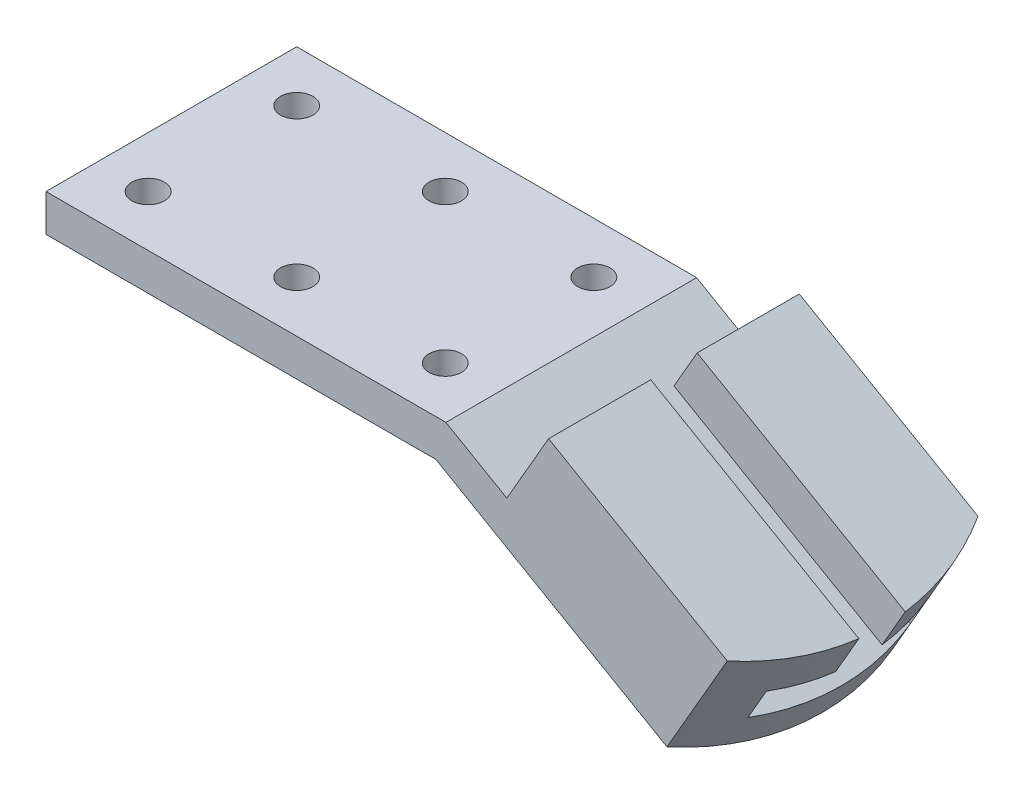
ISO-10303-21;
HEADER;
FILE_DESCRIPTION(('STEP AP214'),'2;1');
FILE_NAME('part.step','',(''),(''),'','','');
FILE_SCHEMA(('AUTOMOTIVE_DESIGN { 1 0 10303 214 1 1 1 1 }'));
ENDSEC;
DATA;
#1=APPLICATION_CONTEXT('core data for automotive mechanical design processes');
#2=APPLICATION_PROTOCOL_DEFINITION('international standard','automotive_design',2000,#1);
#3=PRODUCT_CONTEXT('',#1,'mechanical');
#4=PRODUCT('Part','Part','',(#3));
#5=PRODUCT_RELATED_PRODUCT_CATEGORY('part','',(#4));
#6=PRODUCT_DEFINITION_FORMATION('','',#4);
#7=PRODUCT_DEFINITION_CONTEXT('part definition',#1,'design');
#8=PRODUCT_DEFINITION('design','',#6,#7);
#9=PRODUCT_DEFINITION_SHAPE('','',#8);
#10=(LENGTH_UNIT() NAMED_UNIT(*) SI_UNIT(.MILLI.,.METRE.));
#11=(NAMED_UNIT(*) PLANE_ANGLE_UNIT() SI_UNIT($,.RADIAN.));
#12=(NAMED_UNIT(*) SI_UNIT($,.STERADIAN.) SOLID_ANGLE_UNIT());
#13=UNCERTAINTY_MEASURE_WITH_UNIT(LENGTH_MEASURE(1.E-05),#10,'distance_accuracy_value','');
#14=(GEOMETRIC_REPRESENTATION_CONTEXT(3) GLOBAL_UNCERTAINTY_ASSIGNED_CONTEXT((#13)) GLOBAL_UNIT_ASSIGNED_CONTEXT((#10,
#11,#12)) REPRESENTATION_CONTEXT('',''));
#15=CARTESIAN_POINT('',(0.,0.,0.));
#16=DIRECTION('',(0.,0.,1.));
#17=DIRECTION('',(1.,0.,0.));
#18=AXIS2_PLACEMENT_3D('',#15,#16,#17);
#19=CARTESIAN_POINT('',(25.0000000000001,43.301270189222,27.));
#20=DIRECTION('',(-0.500000000000001,-0.866025403784438,0.));
#21=DIRECTION('',(0.866025403784438,-0.500000000000001,0.));
#22=AXIS2_PLACEMENT_3D('',#19,#20,#21);
#23=PLANE('',#22);
#24=DIRECTION('',(0.866025403784439,-0.5,0.));
#25=VECTOR('',#24,1.);
#26=CARTESIAN_POINT('',(97.5262794416288,1.4282032302755,17.5));
#27=LINE('',#26,#25);
#28=CARTESIAN_POINT('',(99.2583302491977,0.428203230275488,17.5));
#29=VERTEX_POINT('',#28);
#30=CARTESIAN_POINT('',(141.664845078879,-24.055209522035,17.5));
#31=VERTEX_POINT('',#30);
#32=EDGE_CURVE('E246',#29,#31,#27,.T.);
#33=ORIENTED_EDGE('',*,*,#32,.T.);
#34=CARTESIAN_POINT('',(99.2583302491977,0.428203230275488,0.));
#35=DIRECTION('',(-0.500000000000001,-0.866025403784438,0.));
#36=DIRECTION('',(0.866025403784438,-0.500000000000001,0.));
#37=AXIS2_PLACEMENT_3D('',#34,#35,#36);
#38=CIRCLE('',#37,52.);
#39=CARTESIAN_POINT('',(141.664845078879,-24.055209522035,-17.5));
#40=VERTEX_POINT('',#39);
#41=EDGE_CURVE('E220',#31,#40,#38,.F.);
#42=ORIENTED_EDGE('',*,*,#41,.T.);
#43=DIRECTION('',(0.866025403784439,-0.5,0.));
#44=VECTOR('',#43,1.);
#45=CARTESIAN_POINT('',(97.5262794416288,1.4282032302755,-17.5));
#46=LINE('',#45,#44);
#47=CARTESIAN_POINT('',(99.2583302491977,0.428203230275488,-17.5));
#48=VERTEX_POINT('',#47);
#49=EDGE_CURVE('E245',#48,#40,#46,.T.);
#50=ORIENTED_EDGE('',*,*,#49,.F.);
#51=DIRECTION('',(0.,0.,-1.));
#52=VECTOR('',#51,1.);
#53=CARTESIAN_POINT('',(99.2583302491977,0.428203230275481,27.));
#54=LINE('',#53,#52);
#55=CARTESIAN_POINT('',(99.2583302491977,0.428203230275481,-27.));
#56=VERTEX_POINT('',#55);
#57=EDGE_CURVE('E168',#48,#56,#54,.T.);
#58=ORIENTED_EDGE('',*,*,#57,.T.);
#59=DIRECTION('',(-0.866025403784438,0.500000000000001,0.));
#60=VECTOR('',#59,1.);
#61=CARTESIAN_POINT('',(25.0000000000001,43.301270189222,-27.));
#62=LINE('',#61,#60);
#63=CARTESIAN_POINT('',(86.143593539449,8.,-27.));
#64=VERTEX_POINT('',#63);
#65=EDGE_CURVE('E146',#56,#64,#62,.T.);
#66=ORIENTED_EDGE('',*,*,#65,.T.);
#67=DIRECTION('',(0.,0.,-1.));
#68=VECTOR('',#67,1.);
#69=CARTESIAN_POINT('',(86.143593539449,8.,27.));
#70=LINE('',#69,#68);
#71=CARTESIAN_POINT('',(86.143593539449,8.,27.));
#72=VERTEX_POINT('',#71);
#73=EDGE_CURVE('E169',#72,#64,#70,.T.);
#74=ORIENTED_EDGE('',*,*,#73,.F.);
#75=DIRECTION('',(-0.866025403784438,0.500000000000001,0.));
#76=VECTOR('',#75,1.);
#77=CARTESIAN_POINT('',(25.0000000000001,43.301270189222,27.));
#78=LINE('',#77,#76);
#79=CARTESIAN_POINT('',(99.2583302491977,0.428203230275481,27.));
#80=VERTEX_POINT('',#79);
#81=EDGE_CURVE('E103',#80,#72,#78,.T.);
#82=ORIENTED_EDGE('',*,*,#81,.F.);
#83=EDGE_CURVE('E172',#80,#29,#54,.T.);
#84=ORIENTED_EDGE('',*,*,#83,.T.);
#85=EDGE_LOOP('',(#33,#42,#50,#58,#66,#74,#82,#84));
#86=FACE_BOUND('',#85,.T.);
#87=ADVANCED_FACE('F41',(#86),#23,.F.);
#88=CARTESIAN_POINT('',(101.526279441629,8.35640646055095,17.5));
#89=DIRECTION('',(0.5,0.866025403784439,0.));
#90=DIRECTION('',(-0.866025403784439,0.5,0.));
#91=AXIS2_PLACEMENT_3D('',#88,#89,#90);
#92=PLANE('',#91);
#93=DIRECTION('',(0.866025403784439,-0.5,0.));
#94=VECTOR('',#93,1.);
#95=CARTESIAN_POINT('',(101.526279441629,8.35640646055095,5.));
#96=LINE('',#95,#94);
#97=CARTESIAN_POINT('',(103.258330249198,7.35640646055095,5.));
#98=VERTEX_POINT('',#97);
#99=CARTESIAN_POINT('',(148.082988641649,-18.5231221286641,5.));
#100=VERTEX_POINT('',#99);
#101=EDGE_CURVE('E232',#98,#100,#96,.T.);
#102=ORIENTED_EDGE('',*,*,#101,.T.);
#103=CARTESIAN_POINT('',(103.258330249198,7.35640646055096,0.));
#104=DIRECTION('',(0.5,0.866025403784439,0.));
#105=DIRECTION('',(-0.866025403784439,0.5,0.));
#106=AXIS2_PLACEMENT_3D('',#103,#104,#105);
#107=CIRCLE('',#106,52.);
#108=CARTESIAN_POINT('',(145.664845078879,-17.1270062917595,17.5));
#109=VERTEX_POINT('',#108);
#110=EDGE_CURVE('E230',#100,#109,#107,.F.);
#111=ORIENTED_EDGE('',*,*,#110,.T.);
#112=DIRECTION('',(0.866025403784439,-0.5,0.));
#113=VECTOR('',#112,1.);
#114=CARTESIAN_POINT('',(101.526279441629,8.35640646055095,17.5));
#115=LINE('',#114,#113);
#116=CARTESIAN_POINT('',(103.258330249198,7.35640646055095,17.5));
#117=VERTEX_POINT('',#116);
#118=EDGE_CURVE('E221',#117,#109,#115,.T.);
#119=ORIENTED_EDGE('',*,*,#118,.F.);
#120=DIRECTION('',(0.,0.,1.));
#121=VECTOR('',#120,1.);
#122=CARTESIAN_POINT('',(103.258330249198,7.35640646055095,27.));
#123=LINE('',#122,#121);
#124=EDGE_CURVE('E149',#98,#117,#123,.T.);
#125=ORIENTED_EDGE('',*,*,#124,.F.);
#126=EDGE_LOOP('',(#102,#111,#119,#125));
#127=FACE_BOUND('',#126,.T.);
#128=ADVANCED_FACE('F348',(#127),#92,.F.);
#129=CARTESIAN_POINT('',(101.526279441629,8.35640646055095,-17.5));
#130=DIRECTION('',(0.5,0.866025403784439,0.));
#131=DIRECTION('',(-0.866025403784439,0.5,0.));
#132=AXIS2_PLACEMENT_3D('',#129,#130,#131);
#133=PLANE('',#132);
#134=DIRECTION('',(0.866025403784439,-0.5,0.));
#135=VECTOR('',#134,1.);
#136=CARTESIAN_POINT('',(101.526279441629,8.35640646055095,-17.5));
#137=LINE('',#136,#135);
#138=CARTESIAN_POINT('',(103.258330249198,7.35640646055095,-17.5));
#139=VERTEX_POINT('',#138);
#140=CARTESIAN_POINT('',(145.664845078879,-17.1270062917595,-17.5));
#141=VERTEX_POINT('',#140);
#142=EDGE_CURVE('E238',#139,#141,#137,.T.);
#143=ORIENTED_EDGE('',*,*,#142,.T.);
#144=CARTESIAN_POINT('',(103.258330249198,7.35640646055096,0.));
#145=DIRECTION('',(0.5,0.866025403784439,0.));
#146=DIRECTION('',(-0.866025403784439,0.5,0.));
#147=AXIS2_PLACEMENT_3D('',#144,#145,#146);
#148=CIRCLE('',#147,52.);
#149=CARTESIAN_POINT('',(148.082988641649,-18.5231221286641,-5.));
#150=VERTEX_POINT('',#149);
#151=EDGE_CURVE('E209',#141,#150,#148,.F.);
#152=ORIENTED_EDGE('',*,*,#151,.T.);
#153=DIRECTION('',(0.866025403784439,-0.5,0.));
#154=VECTOR('',#153,1.);
#155=CARTESIAN_POINT('',(101.526279441629,8.35640646055095,-5.));
#156=LINE('',#155,#154);
#157=CARTESIAN_POINT('',(103.258330249198,7.35640646055095,-5.));
#158=VERTEX_POINT('',#157);
#159=EDGE_CURVE('E240',#158,#150,#156,.T.);
#160=ORIENTED_EDGE('',*,*,#159,.F.);
#161=DIRECTION('',(0.,0.,1.));
#162=VECTOR('',#161,1.);
#163=CARTESIAN_POINT('',(103.258330249198,7.35640646055095,27.));
#164=LINE('',#163,#162);
#165=EDGE_CURVE('E265',#139,#158,#164,.T.);
#166=ORIENTED_EDGE('',*,*,#165,.F.);
#167=EDGE_LOOP('',(#143,#152,#160,#166));
#168=FACE_BOUND('',#167,.T.);
#169=ADVANCED_FACE('F327',(#168),#133,.F.);
#170=CARTESIAN_POINT('',(74.2583302491977,-42.8730669589465,27.));
#171=DIRECTION('',(0.866025403784438,-0.500000000000001,0.));
#172=DIRECTION('',(0.500000000000001,0.866025403784438,0.));
#173=AXIS2_PLACEMENT_3D('',#170,#171,#172);
#174=PLANE('',#173);
#175=ORIENTED_EDGE('',*,*,#165,.T.);
#176=DIRECTION('',(0.500000000000001,0.866025403784438,0.));
#177=VECTOR('',#176,1.);
#178=CARTESIAN_POINT('',(74.2583302491977,-42.8730669589465,-5.));
#179=LINE('',#178,#177);
#180=CARTESIAN_POINT('',(108.258330249198,16.0166604983953,-5.));
#181=VERTEX_POINT('',#180);
#182=EDGE_CURVE('E237',#158,#181,#179,.T.);
#183=ORIENTED_EDGE('',*,*,#182,.T.);
#184=DIRECTION('',(0.,0.,-1.));
#185=VECTOR('',#184,1.);
#186=CARTESIAN_POINT('',(108.258330249198,16.0166604983954,27.));
#187=LINE('',#186,#185);
#188=CARTESIAN_POINT('',(108.258330249198,16.0166604983954,-27.));
#189=VERTEX_POINT('',#188);
#190=EDGE_CURVE('E145',#181,#189,#187,.T.);
#191=ORIENTED_EDGE('',*,*,#190,.T.);
#192=DIRECTION('',(-0.500000000000001,-0.866025403784438,0.));
#193=VECTOR('',#192,1.);
#194=CARTESIAN_POINT('',(74.2583302491977,-42.8730669589465,-27.));
#195=LINE('',#194,#193);
#196=EDGE_CURVE('E144',#189,#56,#195,.T.);
#197=ORIENTED_EDGE('',*,*,#196,.T.);
#198=ORIENTED_EDGE('',*,*,#57,.F.);
#199=DIRECTION('',(0.500000000000001,0.866025403784438,0.));
#200=VECTOR('',#199,1.);
#201=CARTESIAN_POINT('',(74.2583302491977,-42.8730669589465,-17.5));
#202=LINE('',#201,#200);
#203=EDGE_CURVE('E259',#48,#139,#202,.T.);
#204=ORIENTED_EDGE('',*,*,#203,.T.);
#205=EDGE_LOOP('',(#175,#183,#191,#197,#198,#204));
#206=FACE_BOUND('',#205,.T.);
#207=ADVANCED_FACE('F335',(#206),#174,.F.);
#208=CARTESIAN_POINT('',(34.,58.8897274573418,27.));
#209=DIRECTION('',(-0.500000000000001,-0.866025403784438,0.));
#210=DIRECTION('',(0.866025403784438,-0.500000000000001,0.));
#211=AXIS2_PLACEMENT_3D('',#208,#209,#210);
#212=PLANE('',#211);
#213=DIRECTION('',(-0.866025403784438,0.500000000000001,0.));
#214=VECTOR('',#213,1.);
#215=CARTESIAN_POINT('',(34.,58.8897274573418,27.));
#216=LINE('',#215,#214);
#217=CARTESIAN_POINT('',(146.745341045049,-6.20382554489359,27.));
#218=VERTEX_POINT('',#217);
#219=CARTESIAN_POINT('',(108.258330249198,16.0166604983954,27.));
#220=VERTEX_POINT('',#219);
#221=EDGE_CURVE('E66',#218,#220,#216,.T.);
#222=ORIENTED_EDGE('',*,*,#221,.F.);
#223=CARTESIAN_POINT('',(108.258330249198,16.0166604983954,0.));
#224=DIRECTION('',(-0.500000000000001,-0.866025403784438,0.));
#225=DIRECTION('',(-0.866025403784438,0.500000000000001,0.));
#226=AXIS2_PLACEMENT_3D('',#223,#224,#225);
#227=CIRCLE('',#226,52.);
#228=CARTESIAN_POINT('',(153.082988641649,-9.86286809081971,5.));
#229=VERTEX_POINT('',#228);
#230=EDGE_CURVE('E194',#229,#218,#227,.T.);
#231=ORIENTED_EDGE('',*,*,#230,.F.);
#232=DIRECTION('',(-0.866025403784438,0.500000000000001,0.));
#233=VECTOR('',#232,1.);
#234=CARTESIAN_POINT('',(34.,58.8897274573418,5.));
#235=LINE('',#234,#233);
#236=CARTESIAN_POINT('',(108.258330249198,16.0166604983953,5.));
#237=VERTEX_POINT('',#236);
#238=EDGE_CURVE('E49',#229,#237,#235,.T.);
#239=ORIENTED_EDGE('',*,*,#238,.T.);
#240=EDGE_CURVE('E162',#220,#237,#187,.T.);
#241=ORIENTED_EDGE('',*,*,#240,.F.);
#242=EDGE_LOOP('',(#222,#231,#239,#241));
#243=FACE_BOUND('',#242,.T.);
#244=ADVANCED_FACE('F345',(#243),#212,.F.);
#245=ORIENTED_EDGE('',*,*,#240,.T.);
#246=DIRECTION('',(-0.500000000000001,-0.866025403784438,0.));
#247=VECTOR('',#246,1.);
#248=CARTESIAN_POINT('',(74.2583302491977,-42.8730669589465,5.));
#249=LINE('',#248,#247);
#250=EDGE_CURVE('E251',#237,#98,#249,.T.);
#251=ORIENTED_EDGE('',*,*,#250,.T.);
#252=ORIENTED_EDGE('',*,*,#124,.T.);
#253=DIRECTION('',(-0.500000000000001,-0.866025403784438,0.));
#254=VECTOR('',#253,1.);
#255=CARTESIAN_POINT('',(74.2583302491977,-42.8730669589465,17.5));
#256=LINE('',#255,#254);
#257=EDGE_CURVE('E258',#117,#29,#256,.T.);
#258=ORIENTED_EDGE('',*,*,#257,.T.);
#259=ORIENTED_EDGE('',*,*,#83,.F.);
#260=DIRECTION('',(-0.500000000000001,-0.866025403784438,0.));
#261=VECTOR('',#260,1.);
#262=CARTESIAN_POINT('',(74.2583302491977,-42.8730669589465,27.));
#263=LINE('',#262,#261);
#264=EDGE_CURVE('E165',#220,#80,#263,.T.);
#265=ORIENTED_EDGE('',*,*,#264,.F.);
#266=EDGE_LOOP('',(#245,#251,#252,#258,#259,#265));
#267=FACE_BOUND('',#266,.T.);
#268=ADVANCED_FACE('F43',(#267),#174,.F.);
#269=CARTESIAN_POINT('',(0.,8.,27.));
#270=DIRECTION('',(0.,1.,0.));
#271=DIRECTION('',(0.,0.,1.));
#272=AXIS2_PLACEMENT_3D('',#269,#270,#271);
#273=PLANE('',#272);
#274=CARTESIAN_POINT('',(43.,8.,-16.));
#275=DIRECTION('',(0.,1.,0.));
#276=DIRECTION('',(0.,0.,1.));
#277=AXIS2_PLACEMENT_3D('',#274,#275,#276);
#278=CIRCLE('',#277,3.50000000000001);
#279=CARTESIAN_POINT('',(43.,8.,-12.5));
#280=VERTEX_POINT('',#279);
#281=EDGE_CURVE('E382',#280,#280,#278,.T.);
#282=ORIENTED_EDGE('',*,*,#281,.F.);
#283=EDGE_LOOP('',(#282));
#284=FACE_BOUND('',#283,.T.);
#285=CARTESIAN_POINT('',(75.,8.,-16.));
#286=DIRECTION('',(0.,1.,0.));
#287=DIRECTION('',(0.,0.,1.));
#288=AXIS2_PLACEMENT_3D('',#285,#286,#287);
#289=CIRCLE('',#288,3.50000000000001);
#290=CARTESIAN_POINT('',(75.,8.,-12.5));
#291=VERTEX_POINT('',#290);
#292=EDGE_CURVE('E390',#291,#291,#289,.T.);
#293=ORIENTED_EDGE('',*,*,#292,.F.);
#294=EDGE_LOOP('',(#293));
#295=FACE_BOUND('',#294,.T.);
#296=CARTESIAN_POINT('',(11.0000000000003,8.,16.));
#297=DIRECTION('',(0.,1.,0.));
#298=DIRECTION('',(0.,0.,1.));
#299=AXIS2_PLACEMENT_3D('',#296,#297,#298);
#300=CIRCLE('',#299,3.5);
#301=CARTESIAN_POINT('',(11.0000000000003,8.,19.5));
#302=VERTEX_POINT('',#301);
#303=EDGE_CURVE('E392',#302,#302,#300,.T.);
#304=ORIENTED_EDGE('',*,*,#303,.F.);
#305=EDGE_LOOP('',(#304));
#306=FACE_BOUND('',#305,.T.);
#307=CARTESIAN_POINT('',(43.0000000000003,8.,16.));
#308=DIRECTION('',(0.,1.,0.));
#309=DIRECTION('',(0.,0.,1.));
#310=AXIS2_PLACEMENT_3D('',#307,#308,#309);
#311=CIRCLE('',#310,3.50000000000001);
#312=CARTESIAN_POINT('',(43.0000000000003,8.,19.5));
#313=VERTEX_POINT('',#312);
#314=EDGE_CURVE('E393',#313,#313,#311,.T.);
#315=ORIENTED_EDGE('',*,*,#314,.F.);
#316=EDGE_LOOP('',(#315));
#317=FACE_BOUND('',#316,.T.);
#318=CARTESIAN_POINT('',(75.0000000000003,8.,16.));
#319=DIRECTION('',(0.,1.,0.));
#320=DIRECTION('',(0.,0.,1.));
#321=AXIS2_PLACEMENT_3D('',#318,#319,#320);
#322=CIRCLE('',#321,3.50000000000001);
#323=CARTESIAN_POINT('',(75.0000000000003,8.,19.5));
#324=VERTEX_POINT('',#323);
#325=EDGE_CURVE('E398',#324,#324,#322,.T.);
#326=ORIENTED_EDGE('',*,*,#325,.F.);
#327=EDGE_LOOP('',(#326));
#328=FACE_BOUND('',#327,.T.);
#329=CARTESIAN_POINT('',(11.,8.,-16.));
#330=DIRECTION('',(0.,1.,0.));
#331=DIRECTION('',(0.,0.,1.));
#332=AXIS2_PLACEMENT_3D('',#329,#330,#331);
#333=CIRCLE('',#332,3.5);
#334=CARTESIAN_POINT('',(11.,8.,-12.5));
#335=VERTEX_POINT('',#334);
#336=EDGE_CURVE('E185',#335,#335,#333,.T.);
#337=ORIENTED_EDGE('',*,*,#336,.F.);
#338=EDGE_LOOP('',(#337));
#339=FACE_BOUND('',#338,.T.);
#340=DIRECTION('',(1.,0.,0.));
#341=VECTOR('',#340,1.);
#342=CARTESIAN_POINT('',(0.,8.,-27.));
#343=LINE('',#342,#341);
#344=CARTESIAN_POINT('',(0.,8.,-27.));
#345=VERTEX_POINT('',#344);
#346=EDGE_CURVE('E155',#345,#64,#343,.T.);
#347=ORIENTED_EDGE('',*,*,#346,.F.);
#348=DIRECTION('',(0.,0.,-1.));
#349=VECTOR('',#348,1.);
#350=CARTESIAN_POINT('',(0.,8.,27.));
#351=LINE('',#350,#349);
#352=CARTESIAN_POINT('',(0.,8.,27.));
#353=VERTEX_POINT('',#352);
#354=EDGE_CURVE('E122',#353,#345,#351,.T.);
#355=ORIENTED_EDGE('',*,*,#354,.F.);
#356=DIRECTION('',(1.,0.,0.));
#357=VECTOR('',#356,1.);
#358=CARTESIAN_POINT('',(0.,8.,27.));
#359=LINE('',#358,#357);
#360=EDGE_CURVE('E140',#353,#72,#359,.T.);
#361=ORIENTED_EDGE('',*,*,#360,.T.);
#362=ORIENTED_EDGE('',*,*,#73,.T.);
#363=EDGE_LOOP('',(#347,#355,#361,#362));
#364=FACE_BOUND('',#363,.T.);
#365=ADVANCED_FACE('F275',(#284,#295,#306,#317,#328,#339,#364),#273,.T.);
#366=CARTESIAN_POINT('',(0.,0.,27.));
#367=DIRECTION('',(-1.,0.,0.));
#368=DIRECTION('',(0.,0.,1.));
#369=AXIS2_PLACEMENT_3D('',#366,#367,#368);
#370=PLANE('',#369);
#371=DIRECTION('',(0.,1.,0.));
#372=VECTOR('',#371,1.);
#373=CARTESIAN_POINT('',(0.,0.,-27.));
#374=LINE('',#373,#372);
#375=CARTESIAN_POINT('',(0.,0.,-27.));
#376=VERTEX_POINT('',#375);
#377=EDGE_CURVE('E118',#376,#345,#374,.T.);
#378=ORIENTED_EDGE('',*,*,#377,.F.);
#379=DIRECTION('',(0.,0.,-1.));
#380=VECTOR('',#379,1.);
#381=CARTESIAN_POINT('',(0.,0.,27.));
#382=LINE('',#381,#380);
#383=CARTESIAN_POINT('',(0.,0.,27.));
#384=VERTEX_POINT('',#383);
#385=EDGE_CURVE('E111',#384,#376,#382,.T.);
#386=ORIENTED_EDGE('',*,*,#385,.F.);
#387=DIRECTION('',(0.,1.,0.));
#388=VECTOR('',#387,1.);
#389=CARTESIAN_POINT('',(0.,0.,27.));
#390=LINE('',#389,#388);
#391=EDGE_CURVE('E120',#384,#353,#390,.T.);
#392=ORIENTED_EDGE('',*,*,#391,.T.);
#393=ORIENTED_EDGE('',*,*,#354,.T.);
#394=EDGE_LOOP('',(#378,#386,#392,#393));
#395=FACE_BOUND('',#394,.T.);
#396=ADVANCED_FACE('F117',(#395),#370,.T.);
#397=CARTESIAN_POINT('',(0.,0.,27.));
#398=DIRECTION('',(0.,1.,0.));
#399=DIRECTION('',(0.,0.,1.));
#400=AXIS2_PLACEMENT_3D('',#397,#398,#399);
#401=PLANE('',#400);
#402=CARTESIAN_POINT('',(43.,0.,-16.));
#403=DIRECTION('',(0.,1.,0.));
#404=DIRECTION('',(0.,0.,1.));
#405=AXIS2_PLACEMENT_3D('',#402,#403,#404);
#406=CIRCLE('',#405,3.50000000000001);
#407=CARTESIAN_POINT('',(43.,0.,-12.5));
#408=VERTEX_POINT('',#407);
#409=EDGE_CURVE('E44',#408,#408,#406,.T.);
#410=ORIENTED_EDGE('',*,*,#409,.T.);
#411=EDGE_LOOP('',(#410));
#412=FACE_BOUND('',#411,.T.);
#413=CARTESIAN_POINT('',(75.,0.,-16.));
#414=DIRECTION('',(0.,1.,0.));
#415=DIRECTION('',(0.,0.,1.));
#416=AXIS2_PLACEMENT_3D('',#413,#414,#415);
#417=CIRCLE('',#416,3.50000000000001);
#418=CARTESIAN_POINT('',(75.,0.,-12.5));
#419=VERTEX_POINT('',#418);
#420=EDGE_CURVE('E188',#419,#419,#417,.T.);
#421=ORIENTED_EDGE('',*,*,#420,.T.);
#422=EDGE_LOOP('',(#421));
#423=FACE_BOUND('',#422,.T.);
#424=CARTESIAN_POINT('',(11.0000000000003,0.,16.));
#425=DIRECTION('',(0.,1.,0.));
#426=DIRECTION('',(0.,0.,1.));
#427=AXIS2_PLACEMENT_3D('',#424,#425,#426);
#428=CIRCLE('',#427,3.5);
#429=CARTESIAN_POINT('',(11.0000000000003,0.,19.5));
#430=VERTEX_POINT('',#429);
#431=EDGE_CURVE('E190',#430,#430,#428,.T.);
#432=ORIENTED_EDGE('',*,*,#431,.T.);
#433=EDGE_LOOP('',(#432));
#434=FACE_BOUND('',#433,.T.);
#435=CARTESIAN_POINT('',(43.0000000000003,0.,16.));
#436=DIRECTION('',(0.,1.,0.));
#437=DIRECTION('',(0.,0.,1.));
#438=AXIS2_PLACEMENT_3D('',#435,#436,#437);
#439=CIRCLE('',#438,3.50000000000001);
#440=CARTESIAN_POINT('',(43.0000000000003,0.,19.5));
#441=VERTEX_POINT('',#440);
#442=EDGE_CURVE('E183',#441,#441,#439,.T.);
#443=ORIENTED_EDGE('',*,*,#442,.T.);
#444=EDGE_LOOP('',(#443));
#445=FACE_BOUND('',#444,.T.);
#446=CARTESIAN_POINT('',(75.0000000000003,0.,16.));
#447=DIRECTION('',(0.,1.,0.));
#448=DIRECTION('',(0.,0.,1.));
#449=AXIS2_PLACEMENT_3D('',#446,#447,#448);
#450=CIRCLE('',#449,3.50000000000001);
#451=CARTESIAN_POINT('',(75.0000000000003,0.,19.5));
#452=VERTEX_POINT('',#451);
#453=EDGE_CURVE('E182',#452,#452,#450,.T.);
#454=ORIENTED_EDGE('',*,*,#453,.T.);
#455=EDGE_LOOP('',(#454));
#456=FACE_BOUND('',#455,.T.);
#457=CARTESIAN_POINT('',(11.,0.,-16.));
#458=DIRECTION('',(0.,1.,0.));
#459=DIRECTION('',(0.,0.,1.));
#460=AXIS2_PLACEMENT_3D('',#457,#458,#459);
#461=CIRCLE('',#460,3.5);
#462=CARTESIAN_POINT('',(11.,0.,-12.5));
#463=VERTEX_POINT('',#462);
#464=EDGE_CURVE('E177',#463,#463,#461,.T.);
#465=ORIENTED_EDGE('',*,*,#464,.T.);
#466=EDGE_LOOP('',(#465));
#467=FACE_BOUND('',#466,.T.);
#468=DIRECTION('',(1.,0.,0.));
#469=VECTOR('',#468,1.);
#470=CARTESIAN_POINT('',(0.,0.,-27.));
#471=LINE('',#470,#469);
#472=CARTESIAN_POINT('',(84.,0.,-27.));
#473=VERTEX_POINT('',#472);
#474=EDGE_CURVE('E156',#376,#473,#471,.T.);
#475=ORIENTED_EDGE('',*,*,#474,.T.);
#476=DIRECTION('',(0.,0.,-1.));
#477=VECTOR('',#476,1.);
#478=CARTESIAN_POINT('',(84.,0.,27.));
#479=LINE('',#478,#477);
#480=CARTESIAN_POINT('',(84.,0.,27.));
#481=VERTEX_POINT('',#480);
#482=EDGE_CURVE('E123',#481,#473,#479,.T.);
#483=ORIENTED_EDGE('',*,*,#482,.F.);
#484=DIRECTION('',(1.,0.,0.));
#485=VECTOR('',#484,1.);
#486=CARTESIAN_POINT('',(0.,0.,27.));
#487=LINE('',#486,#485);
#488=EDGE_CURVE('E130',#384,#481,#487,.T.);
#489=ORIENTED_EDGE('',*,*,#488,.F.);
#490=ORIENTED_EDGE('',*,*,#385,.T.);
#491=EDGE_LOOP('',(#475,#483,#489,#490));
#492=FACE_BOUND('',#491,.T.);
#493=ADVANCED_FACE('F126',(#412,#423,#434,#445,#456,#467,#492),#401,.F.);
#494=CARTESIAN_POINT('',(21.0000000000001,36.3730669589465,27.));
#495=DIRECTION('',(0.500000000000001,0.866025403784438,0.));
#496=DIRECTION('',(-0.866025403784438,0.500000000000001,0.));
#497=AXIS2_PLACEMENT_3D('',#494,#495,#496);
#498=PLANE('',#497);
#499=DIRECTION('',(0.866025403784438,-0.500000000000001,0.));
#500=VECTOR('',#499,1.);
#501=CARTESIAN_POINT('',(21.0000000000001,36.3730669589465,-27.));
#502=LINE('',#501,#500);
#503=CARTESIAN_POINT('',(133.745341045049,-28.720486043289,-27.));
#504=VERTEX_POINT('',#503);
#505=EDGE_CURVE('E158',#473,#504,#502,.T.);
#506=ORIENTED_EDGE('',*,*,#505,.T.);
#507=CARTESIAN_POINT('',(95.2583302491977,-6.50000000000001,0.));
#508=DIRECTION('',(0.500000000000001,0.866025403784438,0.));
#509=DIRECTION('',(-0.866025403784438,0.500000000000001,0.));
#510=AXIS2_PLACEMENT_3D('',#507,#508,#509);
#511=CIRCLE('',#510,52.);
#512=CARTESIAN_POINT('',(133.745341045049,-28.720486043289,27.));
#513=VERTEX_POINT('',#512);
#514=EDGE_CURVE('E222',#504,#513,#511,.F.);
#515=ORIENTED_EDGE('',*,*,#514,.T.);
#516=DIRECTION('',(0.866025403784438,-0.500000000000001,0.));
#517=VECTOR('',#516,1.);
#518=CARTESIAN_POINT('',(21.0000000000001,36.3730669589465,27.));
#519=LINE('',#518,#517);
#520=EDGE_CURVE('E134',#481,#513,#519,.T.);
#521=ORIENTED_EDGE('',*,*,#520,.F.);
#522=ORIENTED_EDGE('',*,*,#482,.T.);
#523=EDGE_LOOP('',(#506,#515,#521,#522));
#524=FACE_BOUND('',#523,.T.);
#525=ADVANCED_FACE('F279',(#524),#498,.F.);
#526=DIRECTION('',(0.866025403784438,-0.500000000000001,0.));
#527=VECTOR('',#526,1.);
#528=CARTESIAN_POINT('',(34.,58.8897274573418,-5.));
#529=LINE('',#528,#527);
#530=CARTESIAN_POINT('',(153.082988641649,-9.86286809081973,-5.));
#531=VERTEX_POINT('',#530);
#532=EDGE_CURVE('E175',#181,#531,#529,.T.);
#533=ORIENTED_EDGE('',*,*,#532,.T.);
#534=CARTESIAN_POINT('',(146.745341045049,-6.20382554489359,-27.));
#535=VERTEX_POINT('',#534);
#536=EDGE_CURVE('E59',#535,#531,#227,.T.);
#537=ORIENTED_EDGE('',*,*,#536,.F.);
#538=DIRECTION('',(-0.866025403784438,0.500000000000001,0.));
#539=VECTOR('',#538,1.);
#540=CARTESIAN_POINT('',(34.,58.8897274573418,-27.));
#541=LINE('',#540,#539);
#542=EDGE_CURVE('E94',#535,#189,#541,.T.);
#543=ORIENTED_EDGE('',*,*,#542,.T.);
#544=ORIENTED_EDGE('',*,*,#190,.F.);
#545=EDGE_LOOP('',(#533,#537,#543,#544));
#546=FACE_BOUND('',#545,.T.);
#547=ADVANCED_FACE('F361',(#546),#212,.F.);
#548=CARTESIAN_POINT('',(0.,0.,27.));
#549=DIRECTION('',(0.,0.,1.));
#550=DIRECTION('',(1.,0.,0.));
#551=AXIS2_PLACEMENT_3D('',#548,#549,#550);
#552=PLANE('',#551);
#553=DIRECTION('',(0.500000000000001,0.866025403784438,0.));
#554=VECTOR('',#553,1.);
#555=CARTESIAN_POINT('',(119.745341045049,-52.9691973492533,27.));
#556=LINE('',#555,#554);
#557=EDGE_CURVE('E204',#513,#218,#556,.T.);
#558=ORIENTED_EDGE('',*,*,#557,.T.);
#559=ORIENTED_EDGE('',*,*,#221,.T.);
#560=ORIENTED_EDGE('',*,*,#264,.T.);
#561=ORIENTED_EDGE('',*,*,#81,.T.);
#562=ORIENTED_EDGE('',*,*,#360,.F.);
#563=ORIENTED_EDGE('',*,*,#391,.F.);
#564=ORIENTED_EDGE('',*,*,#488,.T.);
#565=ORIENTED_EDGE('',*,*,#520,.T.);
#566=EDGE_LOOP('',(#558,#559,#560,#561,#562,#563,#564,#565));
#567=FACE_BOUND('',#566,.T.);
#568=ADVANCED_FACE('F133',(#567),#552,.T.);
#569=CARTESIAN_POINT('',(0.,0.,-27.));
#570=DIRECTION('',(0.,0.,1.));
#571=DIRECTION('',(1.,0.,0.));
#572=AXIS2_PLACEMENT_3D('',#569,#570,#571);
#573=PLANE('',#572);
#574=ORIENTED_EDGE('',*,*,#542,.F.);
#575=DIRECTION('',(0.500000000000001,0.866025403784438,0.));
#576=VECTOR('',#575,1.);
#577=CARTESIAN_POINT('',(119.745341045049,-52.9691973492533,-27.));
#578=LINE('',#577,#576);
#579=EDGE_CURVE('E208',#504,#535,#578,.T.);
#580=ORIENTED_EDGE('',*,*,#579,.F.);
#581=ORIENTED_EDGE('',*,*,#505,.F.);
#582=ORIENTED_EDGE('',*,*,#474,.F.);
#583=ORIENTED_EDGE('',*,*,#377,.T.);
#584=ORIENTED_EDGE('',*,*,#346,.T.);
#585=ORIENTED_EDGE('',*,*,#65,.F.);
#586=ORIENTED_EDGE('',*,*,#196,.F.);
#587=EDGE_LOOP('',(#574,#580,#581,#582,#583,#584,#585,#586));
#588=FACE_BOUND('',#587,.T.);
#589=ADVANCED_FACE('F273',(#588),#573,.F.);
#590=CARTESIAN_POINT('',(101.526279441629,8.35640646055095,-17.5));
#591=DIRECTION('',(0.,0.,-1.));
#592=DIRECTION('',(-1.,0.,0.));
#593=AXIS2_PLACEMENT_3D('',#590,#591,#592);
#594=PLANE('',#593);
#595=ORIENTED_EDGE('',*,*,#49,.T.);
#596=DIRECTION('',(0.500000000000001,0.866025403784438,0.));
#597=VECTOR('',#596,1.);
#598=CARTESIAN_POINT('',(123.664845078879,-55.2321240582748,-17.5));
#599=LINE('',#598,#597);
#600=EDGE_CURVE('E212',#40,#141,#599,.T.);
#601=ORIENTED_EDGE('',*,*,#600,.T.);
#602=ORIENTED_EDGE('',*,*,#142,.F.);
#603=ORIENTED_EDGE('',*,*,#203,.F.);
#604=EDGE_LOOP('',(#595,#601,#602,#603));
#605=FACE_BOUND('',#604,.T.);
#606=ADVANCED_FACE('F329',(#605),#594,.F.);
#607=CARTESIAN_POINT('',(101.526279441629,8.35640646055095,17.5));
#608=DIRECTION('',(0.,0.,1.));
#609=DIRECTION('',(1.,0.,0.));
#610=AXIS2_PLACEMENT_3D('',#607,#608,#609);
#611=PLANE('',#610);
#612=ORIENTED_EDGE('',*,*,#118,.T.);
#613=DIRECTION('',(0.500000000000001,0.866025403784438,0.));
#614=VECTOR('',#613,1.);
#615=CARTESIAN_POINT('',(123.664845078879,-55.2321240582748,17.5));
#616=LINE('',#615,#614);
#617=EDGE_CURVE('E223',#109,#31,#616,.F.);
#618=ORIENTED_EDGE('',*,*,#617,.T.);
#619=ORIENTED_EDGE('',*,*,#32,.F.);
#620=ORIENTED_EDGE('',*,*,#257,.F.);
#621=EDGE_LOOP('',(#612,#618,#619,#620));
#622=FACE_BOUND('',#621,.T.);
#623=ADVANCED_FACE('F350',(#622),#611,.F.);
#624=CARTESIAN_POINT('',(106.526279441629,17.0166604983953,5.));
#625=DIRECTION('',(0.,0.,1.));
#626=DIRECTION('',(1.,0.,0.));
#627=AXIS2_PLACEMENT_3D('',#624,#625,#626);
#628=PLANE('',#627);
#629=ORIENTED_EDGE('',*,*,#238,.F.);
#630=DIRECTION('',(0.500000000000001,0.866025403784438,0.));
#631=VECTOR('',#630,1.);
#632=CARTESIAN_POINT('',(126.082988641649,-56.6282398951794,5.));
#633=LINE('',#632,#631);
#634=EDGE_CURVE('E219',#229,#100,#633,.F.);
#635=ORIENTED_EDGE('',*,*,#634,.T.);
#636=ORIENTED_EDGE('',*,*,#101,.F.);
#637=ORIENTED_EDGE('',*,*,#250,.F.);
#638=EDGE_LOOP('',(#629,#635,#636,#637));
#639=FACE_BOUND('',#638,.T.);
#640=ADVANCED_FACE('F343',(#639),#628,.F.);
#641=CARTESIAN_POINT('',(106.526279441629,17.0166604983953,-5.));
#642=DIRECTION('',(0.,0.,-1.));
#643=DIRECTION('',(-1.,0.,0.));
#644=AXIS2_PLACEMENT_3D('',#641,#642,#643);
#645=PLANE('',#644);
#646=ORIENTED_EDGE('',*,*,#159,.T.);
#647=DIRECTION('',(0.500000000000001,0.866025403784438,0.));
#648=VECTOR('',#647,1.);
#649=CARTESIAN_POINT('',(126.082988641649,-56.6282398951794,-5.));
#650=LINE('',#649,#648);
#651=EDGE_CURVE('E11',#150,#531,#650,.T.);
#652=ORIENTED_EDGE('',*,*,#651,.T.);
#653=ORIENTED_EDGE('',*,*,#532,.F.);
#654=ORIENTED_EDGE('',*,*,#182,.F.);
#655=EDGE_LOOP('',(#646,#652,#653,#654));
#656=FACE_BOUND('',#655,.T.);
#657=ADVANCED_FACE('F422',(#656),#645,.F.);
#658=CARTESIAN_POINT('',(81.2583302491977,-30.7487113059643,0.));
#659=DIRECTION('',(0.500000000000001,0.866025403784438,0.));
#660=DIRECTION('',(-0.866025403784438,0.500000000000001,0.));
#661=AXIS2_PLACEMENT_3D('',#658,#659,#660);
#662=CYLINDRICAL_SURFACE('',#661,52.);
#663=ORIENTED_EDGE('',*,*,#579,.T.);
#664=ORIENTED_EDGE('',*,*,#536,.T.);
#665=ORIENTED_EDGE('',*,*,#651,.F.);
#666=ORIENTED_EDGE('',*,*,#151,.F.);
#667=ORIENTED_EDGE('',*,*,#600,.F.);
#668=ORIENTED_EDGE('',*,*,#41,.F.);
#669=ORIENTED_EDGE('',*,*,#617,.F.);
#670=ORIENTED_EDGE('',*,*,#110,.F.);
#671=ORIENTED_EDGE('',*,*,#634,.F.);
#672=ORIENTED_EDGE('',*,*,#230,.T.);
#673=ORIENTED_EDGE('',*,*,#557,.F.);
#674=ORIENTED_EDGE('',*,*,#514,.F.);
#675=EDGE_LOOP('',(#663,#664,#665,#666,#667,#668,#669,#670,#671,#672,#673,#674));
#676=FACE_BOUND('',#675,.T.);
#677=ADVANCED_FACE('F339',(#676),#662,.T.);
#678=CARTESIAN_POINT('',(11.,-46.,-16.));
#679=DIRECTION('',(0.,1.,0.));
#680=DIRECTION('',(0.,0.,1.));
#681=AXIS2_PLACEMENT_3D('',#678,#679,#680);
#682=CYLINDRICAL_SURFACE('',#681,3.5);
#683=ORIENTED_EDGE('',*,*,#336,.T.);
#684=EDGE_LOOP('',(#683));
#685=FACE_BOUND('',#684,.T.);
#686=ORIENTED_EDGE('',*,*,#464,.F.);
#687=EDGE_LOOP('',(#686));
#688=FACE_BOUND('',#687,.T.);
#689=ADVANCED_FACE('F413',(#685,#688),#682,.F.);
#690=CARTESIAN_POINT('',(75.0000000000003,-46.,16.));
#691=DIRECTION('',(0.,1.,0.));
#692=DIRECTION('',(0.,0.,1.));
#693=AXIS2_PLACEMENT_3D('',#690,#691,#692);
#694=CYLINDRICAL_SURFACE('',#693,3.50000000000001);
#695=ORIENTED_EDGE('',*,*,#325,.T.);
#696=EDGE_LOOP('',(#695));
#697=FACE_BOUND('',#696,.T.);
#698=ORIENTED_EDGE('',*,*,#453,.F.);
#699=EDGE_LOOP('',(#698));
#700=FACE_BOUND('',#699,.T.);
#701=ADVANCED_FACE('F408',(#697,#700),#694,.F.);
#702=CARTESIAN_POINT('',(43.0000000000003,-46.,16.));
#703=DIRECTION('',(0.,1.,0.));
#704=DIRECTION('',(0.,0.,1.));
#705=AXIS2_PLACEMENT_3D('',#702,#703,#704);
#706=CYLINDRICAL_SURFACE('',#705,3.50000000000001);
#707=ORIENTED_EDGE('',*,*,#314,.T.);
#708=EDGE_LOOP('',(#707));
#709=FACE_BOUND('',#708,.T.);
#710=ORIENTED_EDGE('',*,*,#442,.F.);
#711=EDGE_LOOP('',(#710));
#712=FACE_BOUND('',#711,.T.);
#713=ADVANCED_FACE('F412',(#709,#712),#706,.F.);
#714=CARTESIAN_POINT('',(11.0000000000003,-46.,16.));
#715=DIRECTION('',(0.,1.,0.));
#716=DIRECTION('',(0.,0.,1.));
#717=AXIS2_PLACEMENT_3D('',#714,#715,#716);
#718=CYLINDRICAL_SURFACE('',#717,3.5);
#719=ORIENTED_EDGE('',*,*,#303,.T.);
#720=EDGE_LOOP('',(#719));
#721=FACE_BOUND('',#720,.T.);
#722=ORIENTED_EDGE('',*,*,#431,.F.);
#723=EDGE_LOOP('',(#722));
#724=FACE_BOUND('',#723,.T.);
#725=ADVANCED_FACE('F481',(#721,#724),#718,.F.);
#726=CARTESIAN_POINT('',(75.,-46.,-16.));
#727=DIRECTION('',(0.,1.,0.));
#728=DIRECTION('',(0.,0.,1.));
#729=AXIS2_PLACEMENT_3D('',#726,#727,#728);
#730=CYLINDRICAL_SURFACE('',#729,3.50000000000001);
#731=ORIENTED_EDGE('',*,*,#292,.T.);
#732=EDGE_LOOP('',(#731));
#733=FACE_BOUND('',#732,.T.);
#734=ORIENTED_EDGE('',*,*,#420,.F.);
#735=EDGE_LOOP('',(#734));
#736=FACE_BOUND('',#735,.T.);
#737=ADVANCED_FACE('F487',(#733,#736),#730,.F.);
#738=CARTESIAN_POINT('',(43.,-46.,-16.));
#739=DIRECTION('',(0.,1.,0.));
#740=DIRECTION('',(0.,0.,1.));
#741=AXIS2_PLACEMENT_3D('',#738,#739,#740);
#742=CYLINDRICAL_SURFACE('',#741,3.50000000000001);
#743=ORIENTED_EDGE('',*,*,#281,.T.);
#744=EDGE_LOOP('',(#743));
#745=FACE_BOUND('',#744,.T.);
#746=ORIENTED_EDGE('',*,*,#409,.F.);
#747=EDGE_LOOP('',(#746));
#748=FACE_BOUND('',#747,.T.);
#749=ADVANCED_FACE('F499',(#745,#748),#742,.F.);
#750=CLOSED_SHELL('',(#87,#128,#169,#207,#244,#268,#365,#396,#493,#525,#547,#568,#589,#606,#623,
#640,#657,#677,#689,#701,#713,#725,#737,#749));
#751=MANIFOLD_SOLID_BREP('B2',#750);
#752=ADVANCED_BREP_SHAPE_REPRESENTATION('',(#18,#751),#14);
#753=SHAPE_DEFINITION_REPRESENTATION(#9,#752);
ENDSEC;
END-ISO-10303-21;
